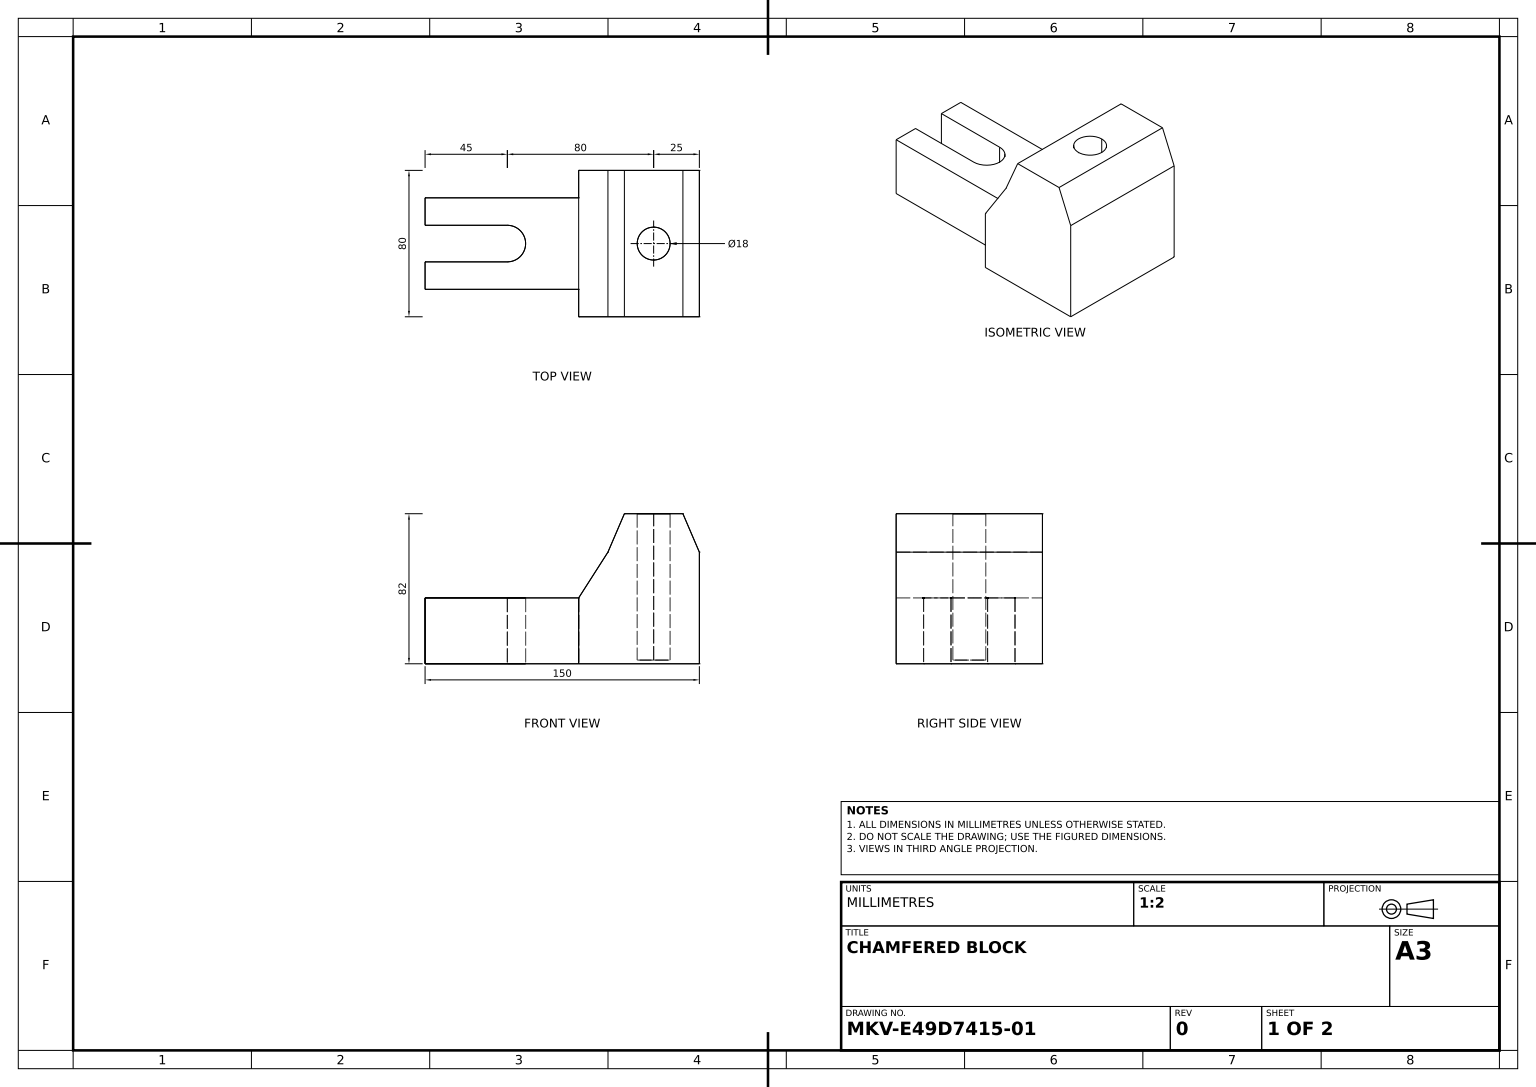
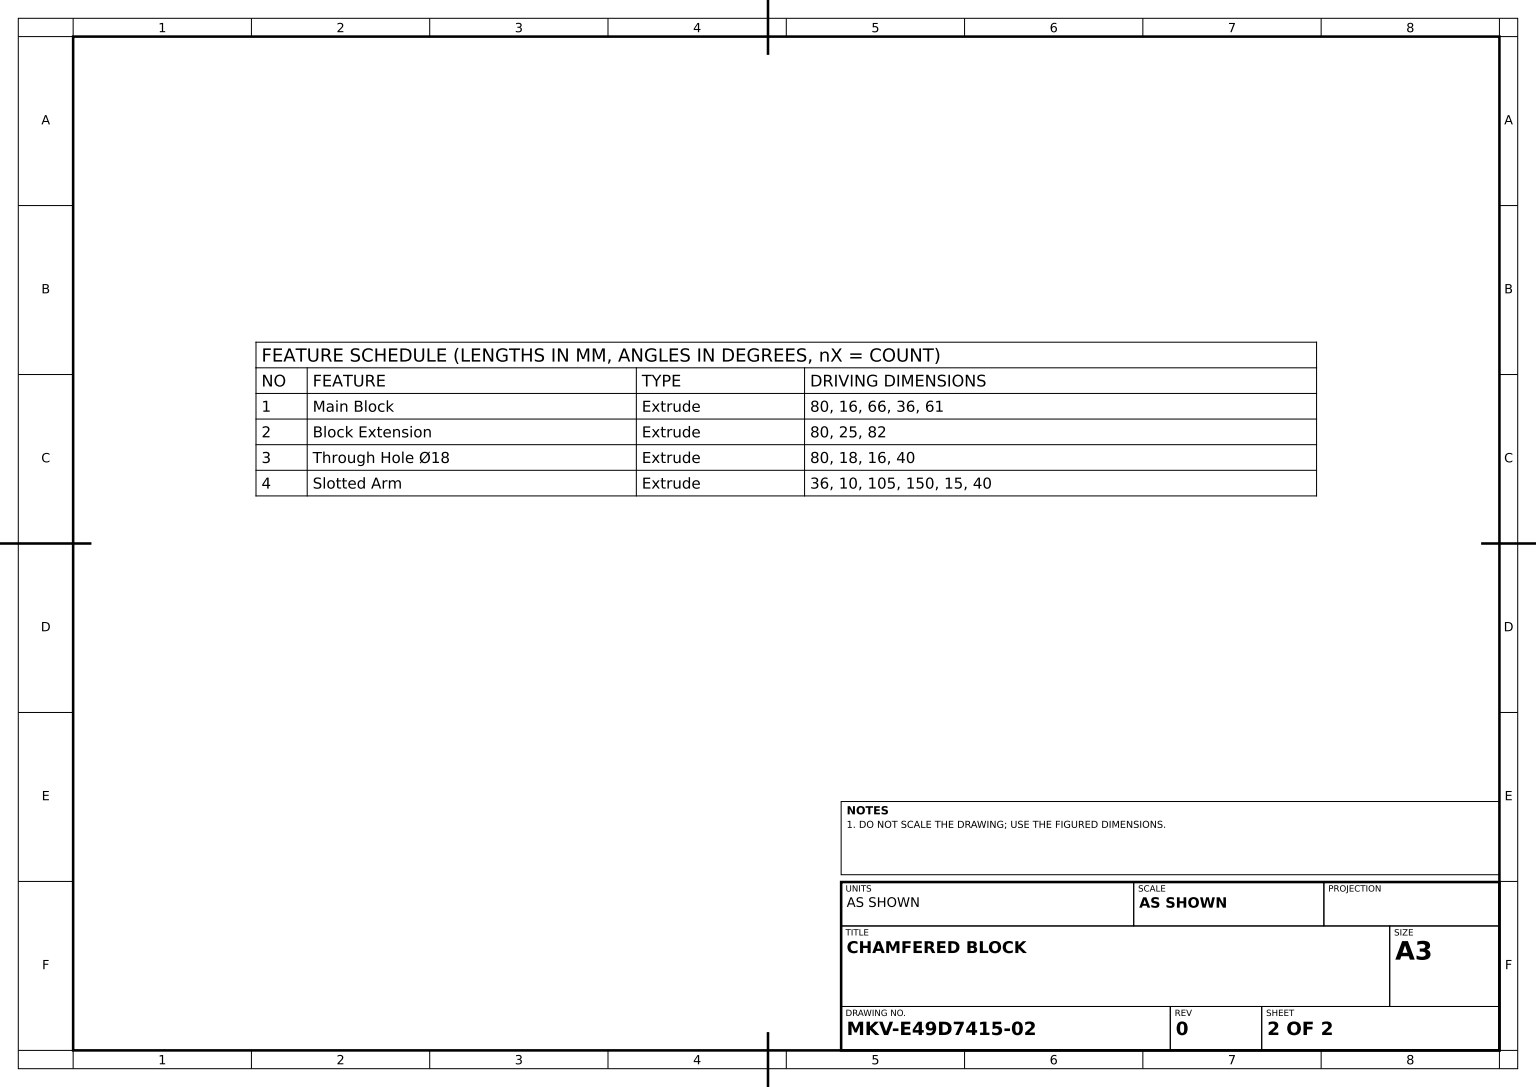
from build123d import *

# Parameters (mm, degrees)
MAIN_BLOCK_DEPTH      = 80
BLOCK_EXTENSION_DEPTH = 80
HOLE_18_SKETCH_R      = 9
THROUGH_HOLE_18_DEPTH = 80
SLOTTED_ARM_DEPTH     = 36


with BuildPart() as part:
    # Main Block Profile → Main Block (new body)
    with BuildSketch(Plane.XY):
        Polygon((0, 0), (66, 0), (66, 61), (16, 61), (0, 36), align=None)
    extrude(amount=MAIN_BLOCK_DEPTH)

    # Block Extension Profile → Block Extension (add)
    with BuildSketch(Plane.XY.offset(80)):
        Polygon((41, 82), (57, 82), (66, 61), (16, 61), (25, 82), align=None)
    extrude(amount=-BLOCK_EXTENSION_DEPTH)

    # Hole Ø18 Sketch → Through Hole Ø18 (cut)
    with BuildSketch(Plane(origin=(0, 82, 0), x_dir=(1, 0, 0), z_dir=(0, 1, 0))):
        with Locations(Location((41, -40, 0), (0, 0, 270))):
            Circle(HOLE_18_SKETCH_R)
    extrude(amount=-THROUGH_HOLE_18_DEPTH, mode=Mode.SUBTRACT)

    # Slotted Arm Profile → Slotted Arm (add)
    with BuildSketch(Plane.XZ):
        with BuildLine():
            Line((0, 65), (0, 15))
            Line((0, 15), (-84, 15))
            Line((-84, 15), (-84, 30))
            Line((-84, 30), (-39, 30))
            ThreePointArc((-39, 30), (-29, 40), (-39, 50))
            Line((-39, 50), (-84, 50))
            Line((-84, 50), (-84, 65))
            Line((-84, 65), (0, 65))
        make_face()
    extrude(amount=-SLOTTED_ARM_DEPTH)


solid = part.part
